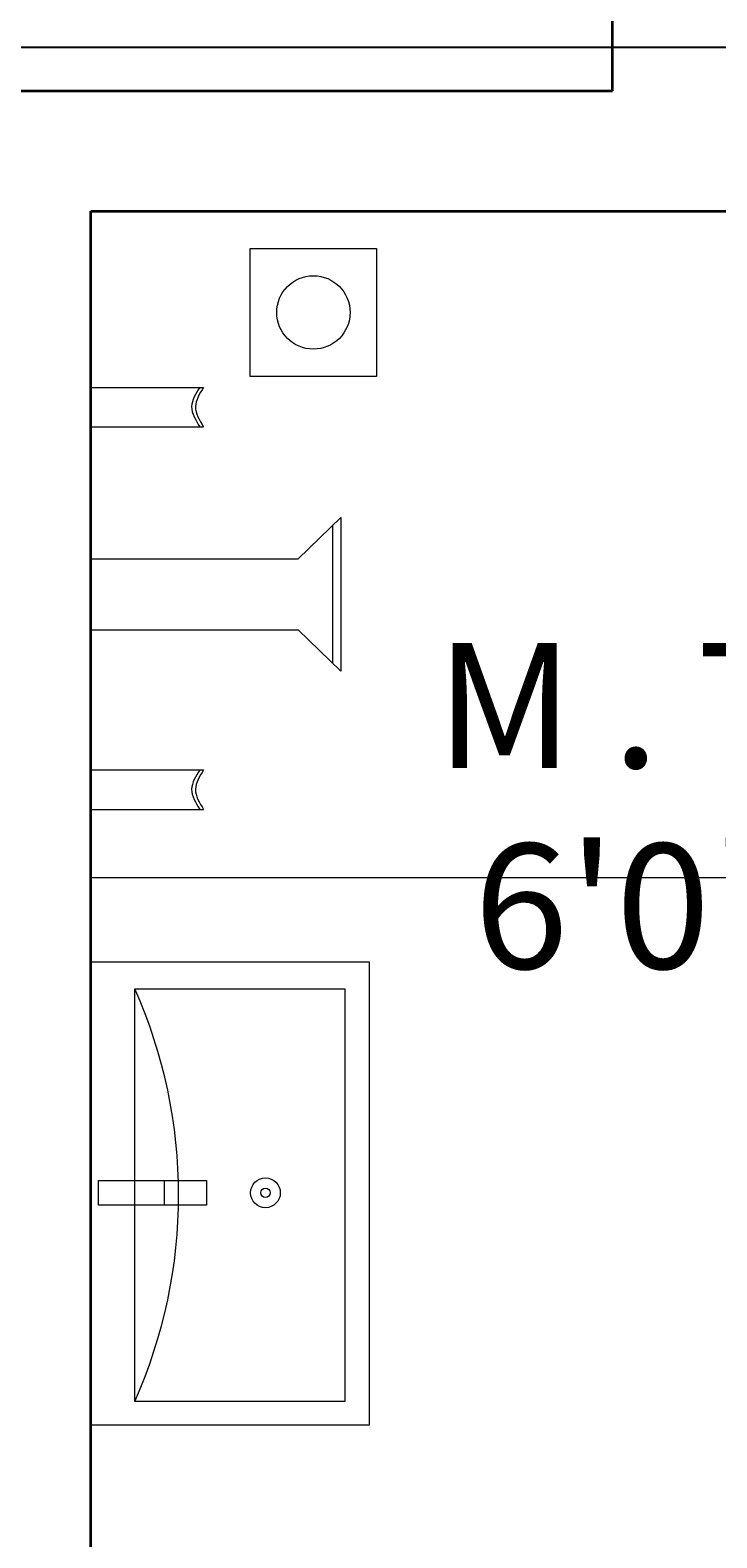
# Model space of a CAD drawing. Units: inches. Extents: x -61 to 1599, y -1316 to 257.
# Tile 61 of 204: x 85 to 119, y -241 to -166. Entities that reach past the tile are written whole.
import ezdxf

# ---------------------------------------------------------------- set-up
doc = ezdxf.new("R2010")
doc.units = ezdxf.units.IN
doc.header["$MEASUREMENT"] = 0
for name, color, linetype, lineweight in [('A-ANNO-DIMS', 2, 'Continuous', 18), ('A-AREA-IDEN', 1, 'Continuous', 18), ('A-FLOR-FIXT', 8, 'Continuous', 18), ('WALLS', 4, 'Continuous', 35)]:
    doc.layers.add(name, color=color, linetype=linetype, lineweight=lineweight)
doc.styles.get("Standard").update_dxf_attribs({"font": 'arial.ttf'})
doc.dimstyles.get("Standard").update_dxf_attribs({"dimtxt": 0.18, "dimasz": 0.18, "dimexe": 0.18, "dimexo": 0.0625, "dimgap": 0.09, "dimtad": 0, "dimtih": 1, "dimtoh": 1, "dimdec": 0, "dimzin": 0, "dimdsep": 46, "dimlunit": 3, "dimtxsty": 'Standard', "dimcen": 0.09, "dimadec": 0, "dimazin": 0, "dimtfac": 1, "dimtdec": 0, "dimtofl": 0, "dimtmove": 0, "dimatfit": 3, "dimfxl": 1, "dimtolj": 1, "dimtzin": 0, "dimarcsym": 0})

# ---------------------------------------------------------------- blocks, each defined once
blk = doc.blocks.new('LAVATORY-WALL-2')
blk.add_line((3.675, 10.958), (3.675, 12.185))
for points in [[(0, 23.069), (13.865, 23.069), (13.865, 0), (0, 0)], [(12.662, 21.727), (12.662, 1.185), (2.198, 1.185), (2.198, 21.727)], [(5.777, 12.185), (5.777, 10.958), (0.396, 10.958), (0.396, 12.185)]]:
    blk.add_lwpolyline(points, close=True)
for radius in [0.74, 0.233]:
    blk.add_circle((8.705, 11.571), radius)
blk.add_arc((-20.864, 11.456), 25.246, 335.99389, 24.00611)
blk = doc.blocks.new('SHOWER-FITTINGS-3')
for p, q in [((0, 21.026), (5.624, 21.026)), ((0, 19.054), (5.624, 19.054)), ((10.338, 12.493), (12.458, 14.542)), ((12.458, 14.542), (12.458, 6.898)), ((12.048, 14.146), (12.048, 7.293)), ((0, 12.493), (10.338, 12.493)), ((0, 8.947), (10.338, 8.947)), ((10.338, 8.947), (12.458, 6.898)), ((0, 1.972), (5.624, 1.972)), ((0, 0), (5.624, 0))]:
    blk.add_line(p, q)
blk.add_lwpolyline([(14.238, 21.574), (7.948, 21.574), (7.948, 27.938), (14.238, 27.938)], close=True)
blk.add_circle((11.093, 24.756), 1.828)
for points in [[(5.435, 21.026), (5.235, 20.706), (4.826, 20.053), (5.229, 19.392), (5.435, 19.054)], [(5.624, 21.026), (5.424, 20.706), (5.016, 20.053), (5.419, 19.392), (5.624, 19.054)], [(5.435, 1.972), (5.235, 1.652), (4.826, 0.998), (5.229, 0.337), (5.435, 0)], [(5.624, 1.972), (5.424, 1.652), (5.016, 0.998), (5.419, 0.337), (5.624, 0)]]:
    blk.add_open_spline(points, degree=3, knots=[0, 0, 0, 0, 1.043806, 2.132489, 2.132489, 2.132489, 2.132489])
blk = doc.blocks.new('*D687')
at = {"layer": 'A-ANNO-DIMS', "color": 0, "lineweight": -2, "transparency": 16777216}
for p, q in [((289.418, 181.677), (-61.077, 181.677)), ((-60.897, 181.497), (-60.897, -528.952)), ((-60.897, -1239.765), (-60.897, -529.316)), ((319.64, -1239.945), (-61.077, -1239.945))]:
    blk.add_line(p, q, dxfattribs=at)
at = {"layer": 'A-ANNO-DIMS', "color": 0, "transparency": 16777216}
for points in [[(-60.927, 181.497), (-60.867, 181.497), (-60.897, 181.677)], [(-60.927, -1239.765), (-60.867, -1239.765), (-60.897, -1239.945)]]:
    blk.add_solid(points, dxfattribs=at)
at = {"layer": 'DEFPOINTS', "color": 0, "transparency": 16777216}
for p in [(289.481, 181.677), (-60.897, -1239.945), (319.703, -1239.945)]:
    blk.add_point(p, dxfattribs=at)
at = {"layer": 'A-ANNO-DIMS', "color": 0, "transparency": 16777216, "insert": (-60.897, -529.134), "char_height": 0.18, "attachment_point": 5}
blk.add_mtext('\\A1;1421.6', dxfattribs=at)
blk = doc.blocks.new('*D699')
at = {"layer": 'A-ANNO-DIMS', "color": 0, "lineweight": -2, "transparency": 16777216}
for p, q in [((835.64, -167.169), (-61.077, -167.169)), ((-60.897, -167.349), (-60.897, -306.726)), ((-60.897, -446.466), (-60.897, -307.09)), ((841.64, -446.646), (-61.077, -446.646))]:
    blk.add_line(p, q, dxfattribs=at)
at = {"layer": 'A-ANNO-DIMS', "color": 0, "transparency": 16777216}
for points in [[(-60.927, -167.349), (-60.867, -167.349), (-60.897, -167.169)], [(-60.927, -446.466), (-60.867, -446.466), (-60.897, -446.646)]]:
    blk.add_solid(points, dxfattribs=at)
at = {"layer": 'DEFPOINTS', "color": 0, "transparency": 16777216}
for p in [(835.703, -167.169), (-60.897, -446.646), (841.703, -446.646)]:
    blk.add_point(p, dxfattribs=at)
at = {"layer": 'A-ANNO-DIMS', "color": 0, "transparency": 16777216, "insert": (-60.897, -306.908), "char_height": 0.18, "attachment_point": 5}
blk.add_mtext('\\A1;279.5', dxfattribs=at)
blk = doc.blocks.new('*D700')
at = {"layer": 'A-ANNO-DIMS', "color": 0, "lineweight": -2, "transparency": 16777216}
for p, q in [((14.703, -616.882), (14.703, 257.457)), ((14.883, 257.277), (96.772, 257.277)), ((179.572, 257.277), (97.683, 257.277)), ((179.752, -616.882), (179.752, 257.457))]:
    blk.add_line(p, q, dxfattribs=at)
at = {"layer": 'A-ANNO-DIMS', "color": 0, "transparency": 16777216}
for points in [[(14.883, 257.307), (14.883, 257.247), (14.703, 257.277)], [(179.572, 257.307), (179.572, 257.247), (179.752, 257.277)]]:
    blk.add_solid(points, dxfattribs=at)
at = {"layer": 'DEFPOINTS', "color": 0, "transparency": 16777216}
for p in [(179.752, 257.277), (14.703, -616.945), (179.752, -616.945)]:
    blk.add_point(p, dxfattribs=at)
at = {"layer": 'A-ANNO-DIMS', "color": 0, "transparency": 16777216, "insert": (97.227, 257.277), "char_height": 0.18, "attachment_point": 5}
blk.add_mtext('\\A1;165.05', dxfattribs=at)

msp = doc.modelspace()

# ---------------------------------------------------------------- linework, layer by layer
at = {"layer": 'A-FLOR-FIXT'}
msp.add_line((87.7028, -208.5091), (159.7028, -208.5091), dxfattribs=at)
at = {"layer": 'WALLS'}
for p, q in [((113.7028, -169.3229), (113.7028, -13.3229)), ((23.7028, -169.3229), (113.7028, -169.3229)), ((87.7028, -282.3229), (87.7028, -175.3229)), ((87.7028, -175.3229), (159.7028, -175.3229))]:
    msp.add_line(p, q, dxfattribs=at)

# ---------------------------------------------------------------- block references
at = {"layer": 'A-FLOR-FIXT'}
for name, p in [('SHOWER-FITTINGS-3', (87.703, -205.124)), ('LAVATORY-WALL-2', (87.703, -235.784))]:
    msp.add_blockref(name, p, dxfattribs=at)

# ---------------------------------------------------------------- texts
at = {"layer": 'A-AREA-IDEN'}
for s, p in [(' M . TOILET', (102.978, -203.0507)), ('  6\'0" X 8\'11"', (102.978, -213.0484))]:
    msp.add_text(s, height=6.223643, dxfattribs=at).set_placement(p)

# ---------------------------------------------------------------- dimensions: what is measured, and where the dimension line sits
at = {"layer": 'A-ANNO-DIMS'}
dim = msp.add_linear_dim(base=(179.7521, 257.2771), p1=(14.7028, -616.9446), p2=(179.7521, -616.9446), dimstyle='Standard', override={"dimdec": 2, "dimlfac": 1, "dimrnd": 0, "dimzin": 0, "dimdsep": 46, "dimlunit": 2}, dxfattribs=at)
dim.commit()
dim.dimension.update_dxf_attribs({"geometry": '*D700', "text_midpoint": (97.2274, 257.2771)})
for base, p1, p2, picture, middle in [((-60.8972, -1239.9446), (289.4807, 181.6771), (319.7028, -1239.9446), '*D687', (-60.8972, -529.1337)), ((-60.8972, -446.6462), (835.7028, -167.169), (841.7028, -446.6462), '*D699', (-60.8972, -306.9076))]:
    dim = msp.add_linear_dim(base=base, p1=p1, p2=p2, angle=90, dimstyle='Standard', override={"dimdec": 1, "dimlfac": 1, "dimrnd": 0, "dimzin": 0, "dimdsep": 46, "dimlunit": 2}, dxfattribs=at)
    dim.commit()
    dim.dimension.update_dxf_attribs({"geometry": picture, "text_midpoint": middle})

doc.saveas('drawing.dxf')
